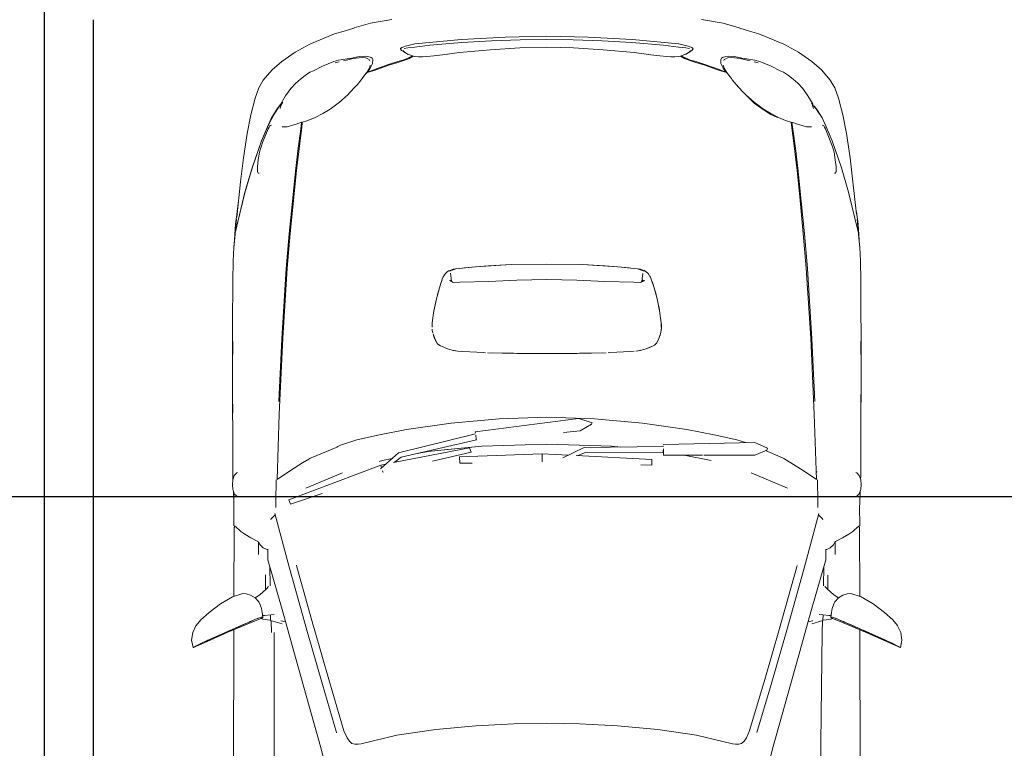
# Model space of a CAD drawing. Units: millimetres. Extents: x 595116 to 630915, y 909473 to 920225.
# Tile 7 of 134: x 629314 to 629404, y 919279 to 919346. Entities that reach past the tile are written whole.
import ezdxf

# ---------------------------------------------------------------- set-up
doc = ezdxf.new("R2010")
doc.units = ezdxf.units.MM
doc.linetypes.add('ACAD_ISO02W100', pattern=[15, 12, -3])
for name, color, linetype, lineweight in [('C-PRKG-VEHI', 8, 'Continuous', 13), ('C-PROP', 7, 'Continuous', 25), ('C-PROP-REF', 240, 'ACAD_ISO02W100', 13), ('Dimension', 3, 'Continuous', 18)]:
    doc.layers.add(name, color=color, linetype=linetype, lineweight=lineweight)
doc.styles.get("Standard").update_dxf_attribs({"font": 'arial.ttf'})
doc.dimstyles.new('ISO-25', dxfattribs={"dimtxt": 9, "dimasz": 6, "dimexe": 1.25, "dimexo": 0.625, "dimtad": 1, "dimlunit": 4, "dimtxsty": 'Standard', "dimcen": 2.5, "dimadec": 0, "dimazin": 0, "dimtfac": 1, "dimtmove": 0, "dimatfit": 3, "dimfxl": 1, "dimarcsym": 0})

# ---------------------------------------------------------------- blocks, each defined once
blk = doc.blocks.new('A$C7ADB3080')
for p, q in [((1725, 1949.3), (1706, 1940.5)), ((1745.5, 1952.4), (1725, 1949.3)), ((1765.9, 1948), (1745.5, 1952.4)), ((1765.8, 1948.2), (1752, 1951)), ((1689.8, 1927.3), (1669.6, 1903.9)), ((1705.6, 1940.3), (1689.8, 1927.3)), ((1706, 1940.5), (1705.6, 1940.3)), ((1750.6, 1917.5), (1752.5, 1921.9)), ((1752.5, 1921.9), (1756.2, 1929.1)), ((1752.5, 1921.9), (1752.5, 1921.9)), ((1765.7, 1947.4), (1752.8, 1918.2)), ((1756.2, 1929.1), (1759.4, 1935.8)), ((1763.8, 1944.5), (1759.4, 1935.8)), ((1759.4, 1935.8), (1762, 1941.3)), ((1759.4, 1935.8), (1759.4, 1935.8)), ((1762, 1941.3), (1763.8, 1944.5)), ((1763.8, 1944.5), (1765, 1946.2)), ((1765, 1946.2), (1765.7, 1947.4)), ((1765.7, 1947.4), (1765.9, 1948)), ((1765.9, 1948), (1765.8, 1948.2)), ((1669.6, 1903.9), (1646.3, 1872.8)), ((1742, 1898.2), (1723, 1855.1)), ((1724.2, 1852.4), (1752.8, 1918.2)), ((1734, 1880.4), (1744, 1903.1)), ((1749.1, 1914.3), (1742, 1898.2)), ((1744, 1903.1), (1746, 1907.5)), ((1746, 1907.5), (1748.3, 1912.5)), ((1748.3, 1912.5), (1750.6, 1917.5)), ((1646.3, 1872.8), (1626.7, 1840.1)), ((1721.5, 1852), (1734, 1880.4)), ((947, 1840.2), (900.9, 1840.1)), ((1014.5, 1840), (947, 1840.2)), ((1724.2, 1852.4), (1697.4, 1788.7)), ((1723, 1855.1), (1704.1, 1812.4)), ((1709.1, 1823.9), (1721.5, 1852)), ((485.6, 1817.6), (419.3, 1809.7)), ((574.5, 1827.8), (485.6, 1817.6)), ((514, 1805.8), (622.7, 1832)), ((568.1, 1827.1), (601.7, 1831.6)), ((596.5, 1830), (587.6, 1828.8)), ((596.5, 1830), (598.5, 1830.3)), ((598.5, 1830.3), (629.8, 1833.4)), ((615.8, 1832.9), (601.7, 1831.6)), ((629.8, 1833.4), (615.8, 1832.9)), ((622.7, 1832), (625.4, 1832.6)), ((625.4, 1832.6), (622.7, 1832)), ((625.4, 1832.6), (627.4, 1832.8)), ((627.4, 1832.8), (625.4, 1832.6)), ((627.4, 1832.8), (629.3, 1833)), ((629.3, 1833), (627.4, 1832.8)), ((630.2, 1833.1), (628.2, 1832.8)), ((644.6, 1834.3), (629.8, 1833.4)), ((666, 1836.1), (630.2, 1833.1)), ((702.2, 1838.3), (666, 1836.1)), ((702.2, 1838.3), (704.4, 1838.4)), ((755.9, 1839.2), (704.4, 1838.4)), ((755.9, 1839.2), (789.1, 1839)), ((846.4, 1839.7), (789.1, 1839)), ((900.9, 1840.1), (846.4, 1839.7)), ((998.4, 1839.9), (923, 1839.2)), ((998.4, 1839.9), (1014.5, 1840)), ((1066.5, 1839.8), (1014.5, 1840)), ((1117.5, 1839.5), (1066.5, 1839.8)), ((1120.4, 1839.3), (1070.3, 1839.6)), ((1164.2, 1839.3), (1117.5, 1839.5)), ((1120.4, 1839.3), (1164.2, 1839.1)), ((1164.2, 1839.1), (1164.1, 1839.1)), ((1186, 1839.2), (1164.2, 1839.3)), ((1211.9, 1839.1), (1164.4, 1839.2)), ((1256.2, 1839), (1211.9, 1839.1)), ((1295.5, 1839), (1256.2, 1839)), ((1284.8, 1825.7), (1285.6, 1828.2)), ((1285.6, 1828.2), (1292.6, 1835.1)), ((1292.6, 1835.1), (1302.3, 1838.5)), ((1295.5, 1839), (1302.9, 1838.7)), ((1302.3, 1838.5), (1304.4, 1839)), ((1304.4, 1839), (1317.7, 1840)), ((1331.1, 1839.1), (1317.7, 1840)), ((1331.1, 1839.1), (1333.2, 1838.5)), ((1342.9, 1835.1), (1333.2, 1838.5)), ((1336.7, 1837.3), (1371.1, 1836.1)), ((1349.8, 1828.2), (1342.9, 1835.1)), ((1350.6, 1825.4), (1349.8, 1828.2)), ((1371.1, 1836.1), (1377.3, 1836)), ((1377.3, 1836), (1430.5, 1836.5)), ((1434.1, 1830.8), (1430.5, 1836.5)), ((1433.4, 1831.8), (1433.4, 1833.5)), ((1433.4, 1833.5), (1433.5, 1833.5)), ((1433.5, 1833.5), (1433.6, 1833.6)), ((1435.6, 1835.7), (1433.6, 1833.6)), ((1445.2, 1818.8), (1434.1, 1830.8)), ((1435.6, 1835.7), (1437, 1835.7)), ((1437, 1835.7), (1625.4, 1836.2)), ((1445.7, 1818.2), (1445.2, 1818.8)), ((1446.6, 1816.9), (1445.7, 1818.2)), ((1453.9, 1805.9), (1446.6, 1816.9)), ((1626.7, 1840.1), (1617.6, 1812)), ((1699.6, 1802.3), (1709.1, 1823.9)), ((1717.5, 1836.5), (2187.9, 1837.4)), ((300.5, 1789.8), (255.3, 1777.9)), ((352.3, 1799.8), (300.5, 1789.8)), ((419.3, 1809.7), (352.3, 1799.8)), ((372.4, 1760.5), (446.6, 1786.3)), ((446.6, 1786.3), (372.4, 1760.5)), ((446.6, 1786.3), (514, 1805.8)), ((514, 1805.8), (446.6, 1786.3)), ((1464, 1789.1), (1453.9, 1805.9)), ((1474.9, 1770), (1464, 1789.1)), ((1617.6, 1812), (1618.4, 1802.1)), ((1618.4, 1802.1), (1622.1, 1790.1)), ((1622.1, 1790.1), (1629.3, 1778)), ((1697.4, 1788.7), (1685.2, 1759.7)), ((1694.1, 1789.9), (1688.5, 1776.5)), ((1691.4, 1783.7), (1694.6, 1791)), ((1691.4, 1783.7), (1694.1, 1789.9)), ((1704.1, 1812.4), (1694.1, 1789.9)), ((1694.1, 1789.9), (1694.6, 1791)), ((1694.6, 1791), (1695.1, 1792.1)), ((1695.1, 1792.1), (1695.6, 1793.4)), ((1695.6, 1793.4), (1696.2, 1794.5)), ((1696.2, 1794.5), (1697.1, 1796.7)), ((1697.1, 1796.7), (1698.1, 1798.8)), ((1698.1, 1798.8), (1698.9, 1800.7)), ((1698.9, 1800.7), (1699.6, 1802.3)), ((227, 1767.4), (205.8, 1755.4)), ((255.3, 1777.9), (227, 1767.4)), ((327.4, 1741.3), (372.4, 1760.5)), ((372.4, 1760.5), (327.4, 1741.3)), ((385.9, 1760.4), (377.1, 1757.2)), ((391.9, 1762.5), (385.9, 1760.4)), ((396.8, 1764.1), (391.9, 1762.5)), ((403.1, 1765.7), (396.8, 1764.1)), ((424.7, 1769.2), (403.1, 1765.7)), ((443.9, 1771.4), (424.7, 1769.2)), ((457.6, 1771.3), (443.9, 1771.4)), ((461, 1769.1), (457.6, 1771.3)), ((461.4, 1766.7), (461, 1769.1)), ((1475.5, 1768.9), (1474.9, 1770)), ((1510, 1768.4), (1475.5, 1768.9)), ((1476.3, 1768.3), (1475.5, 1768.9)), ((1483.6, 1764.1), (1476.3, 1768.3)), ((1491.8, 1755.3), (1483.6, 1764.1)), ((1620.9, 1764.8), (1604.9, 1746.4)), ((1629.8, 1777.6), (1620.9, 1764.8)), ((1629.3, 1778), (1640.8, 1767.9)), ((1640.8, 1767.9), (1649.1, 1763.8)), ((1649.1, 1763.8), (1658.9, 1760.6)), ((1658.9, 1760.6), (1670.1, 1758.3)), ((1683.2, 1763.2), (1682.2, 1758.7)), ((1682.2, 1758.7), (1682.5, 1760.9)), ((1682.5, 1760.9), (1683.2, 1763.2)), ((1688.5, 1776.5), (1683.2, 1763.2)), ((1683.2, 1763.2), (1685.6, 1769.3)), ((1684, 1757.5), (1685.2, 1759.7)), ((1685.2, 1759.7), (1684.6, 1758.5)), ((1685.6, 1769.3), (1688.5, 1776.5)), ((1688, 1756.4), (1686.5, 1762.7)), ((1688.5, 1776.5), (1691.4, 1783.7)), ((205.8, 1755.4), (177.4, 1731.2)), ((296.4, 1724.9), (308.8, 1733)), ((308.8, 1733), (296.4, 1724.9)), ((308.8, 1733), (327.4, 1741.3)), ((327.4, 1741.3), (308.8, 1733)), ((329.5, 1733), (330.6, 1736)), ((331.4, 1737.3), (330.6, 1736)), ((334.6, 1739.6), (331.4, 1737.3)), ((339.6, 1742.2), (334.6, 1739.6)), ((377.1, 1757.2), (339.6, 1742.2)), ((1411.9, 1733.6), (1401.3, 1722.8)), ((1414.5, 1734.8), (1411.9, 1733.6)), ((1496.1, 1745.8), (1491.8, 1755.3)), ((1496.8, 1742), (1496.1, 1745.8)), ((1524.8, 1743.1), (1496.6, 1743.1)), ((1661.6, 1703.9), (1524.8, 1743.1)), ((1596, 1736.9), (1543.4, 1737.8)), ((1607.1, 1748.9), (1567, 1748.9)), ((1604.9, 1746.4), (1597.9, 1740.6)), ((1670.1, 1758.3), (1682.7, 1756.6)), ((1675.3, 1725.1), (1675.9, 1734.9)), ((1675.9, 1734.9), (1677.6, 1752)), ((1692, 1735.3), (1676, 1735.6)), ((1677.6, 1752), (1678.3, 1757.2)), ((1682.3, 1757.1), (1682.2, 1758.7)), ((1682.2, 1758.7), (1682.7, 1756.6)), ((1682.7, 1756.6), (1682.3, 1757.1)), ((1682.7, 1756.6), (1684, 1757.5)), ((1683.3, 1756.9), (1682.7, 1756.6)), ((1684, 1757.5), (1683.3, 1756.9)), ((1684.6, 1758.5), (1684, 1757.5)), ((1690, 1743.9), (1688, 1756.4)), ((1690.8, 1736.6), (1690, 1743.9)), ((1690.9, 1735.3), (1690.8, 1736.6)), ((1700.5, 1704.4), (1692, 1735.3)), ((1724.4, 1733.1), (1692.5, 1733.5)), ((2375.6, 1724.9), (1724.4, 1733.1)), ((177.4, 1731.2), (154.5, 1704.8)), ((248.7, 1693.9), (272.8, 1708.2)), ((272.8, 1708.2), (248.7, 1693.9)), ((274.1, 1706.2), (268.7, 1703.4)), ((278, 1711.4), (275.4, 1709.5)), ((275.5, 1706.9), (283.4, 1709.5)), ((276.7, 1711.4), (284.8, 1717.1)), ((287.5, 1718), (278, 1711.4)), ((284.8, 1717.1), (296.4, 1724.9)), ((298.6, 1725.5), (287.5, 1718)), ((1124.1, 1711.4), (915.2, 1701.7)), ((917.2, 1704.7), (1089.1, 1712.9)), ((1303.7, 1717.2), (1124.1, 1711.4)), ((1279.1, 1680.6), (1303.7, 1717.2)), ((1284, 1719.6), (1282.1, 1716.5)), ((1304.9, 1720.3), (1365.2, 1721)), ((1365.2, 1721), (1380.7, 1721.1)), ((1397.7, 1723.7), (1548.1, 1683.7)), ((1692.9, 1707.2), (1693, 1706.9)), ((1693, 1706.9), (1695.6, 1694.4)), ((128.8, 1668.1), (153.9, 1704.5)), ((214.1, 1665.8), (228.3, 1679.7)), ((228.3, 1679.7), (214.1, 1665.8)), ((228.3, 1679.7), (248.7, 1693.9)), ((248.7, 1693.9), (228.3, 1679.7)), ((330.2, 1678.1), (326.2, 1665.2)), ((333.4, 1690.2), (330.2, 1678.1)), ((333.6, 1703.6), (333.4, 1690.2)), ((627.3, 1681.1), (536.8, 1672.6)), ((538.3, 1675.5), (628.6, 1684.1)), ((722.4, 1689.2), (627.3, 1681.1)), ((628.6, 1684.1), (723.6, 1692.3)), ((915.2, 1701.7), (722.4, 1689.2)), ((723.6, 1692.3), (917.2, 1704.7)), ((1257.7, 1647.2), (1279.1, 1680.6)), ((1548.1, 1683.7), (1718.6, 1636)), ((1799.6, 1665.1), (1661.6, 1703.9)), ((106.5, 1627.7), (128.8, 1668.1)), ((192.9, 1640.1), (202.7, 1653)), ((202.7, 1653), (192.9, 1640.1)), ((202.7, 1653), (214.1, 1665.8)), ((214.1, 1665.8), (202.7, 1653)), ((326.2, 1665.2), (320.7, 1650)), ((320.7, 1650), (340.1, 1652.4)), ((343.5, 1650.7), (321.3, 1648)), ((340.1, 1652.4), (392.9, 1659.3)), ((371.1, 1654.1), (343.5, 1650.7)), ((401.8, 1657.9), (371.1, 1654.1)), ((392.9, 1659.3), (455.7, 1666.7)), ((454.1, 1664), (401.8, 1657.9)), ((536.8, 1672.6), (454.1, 1664)), ((455.7, 1666.7), (538.2, 1675.4)), ((538.2, 1675.4), (538.2, 1675.4)), ((538.3, 1675.5), (538.3, 1675.5)), ((1543.7, 1663.2), (1540.2, 1664.1)), ((1714, 1615.6), (1543.7, 1663.2)), ((1927.3, 1629.4), (1799.6, 1665.1)), ((78.4, 1559.2), (106.5, 1627.7)), ((179.4, 1617.7), (183.6, 1626.9)), ((183.6, 1626.9), (179.4, 1617.7)), ((183.6, 1626.9), (192.9, 1640.1)), ((192.9, 1640.1), (183.6, 1626.9)), ((308, 1612.7), (316.4, 1632.4)), ((316.4, 1632.4), (321.9, 1649.9)), ((320.7, 1649.8), (320.7, 1650)), ((320.7, 1650), (321, 1650)), ((321.9, 1649.9), (322, 1650.2)), ((1224.6, 1577), (1244.4, 1624.1)), ((1244.4, 1624.1), (1245.8, 1627.5)), ((1245.8, 1627.5), (1247.6, 1630.5)), ((1247.6, 1630.5), (1257.7, 1647.2)), ((1285.5, 1538), (1327.9, 1638.1)), ((1718.6, 1636), (1868.2, 1592.8)), ((2038.3, 1598.2), (1927.3, 1629.4)), ((166.6, 1592.6), (179.4, 1617.7)), ((179.4, 1617.7), (166.6, 1592.6)), ((297.6, 1592.1), (308, 1612.7)), ((299.6, 1592.1), (308.6, 1609.9)), ((1714, 1615.6), (1708.7, 1617.1)), ((1860.7, 1573.2), (1714, 1615.6)), ((2088.8, 1585.4), (2038.3, 1598.2)), ((154.1, 1561.6), (166.6, 1592.6)), ((166.6, 1592.6), (154.1, 1561.6)), ((265.7, 1546.2), (285.2, 1572)), ((284.8, 1567.7), (299.6, 1592.1)), ((285.2, 1572), (297.6, 1592.1)), ((1201.9, 1547.7), (1217.9, 1583.1)), ((1223, 1580.9), (1217.9, 1583.1)), ((1236.7, 1548.1), (1223, 1580.9)), ((1863.6, 1572.4), (1860.7, 1573.2)), ((1994.6, 1533.7), (1863.6, 1572.4)), ((1868.2, 1592.8), (2000, 1553.9)), ((70.3, 1532.9), (78.4, 1559.2)), ((147.2, 1525.2), (150.6, 1548.3)), ((150.6, 1548.3), (147.2, 1525.2)), ((150.6, 1548.3), (154.1, 1561.6)), ((154.1, 1561.6), (150.6, 1548.3)), ((158.2, 1557.5), (154.9, 1546.4)), ((245.7, 1523), (265.7, 1546.2)), ((268.5, 1546.6), (247.9, 1525.1)), ((284.8, 1567.7), (268.5, 1546.6)), ((284.8, 1567.7), (284.7, 1567.6)), ((1207.6, 1296.6), (1201.9, 1547.7)), ((1236.9, 1407.5), (1236.7, 1548.1)), ((62.1, 1506.7), (66.6, 1521)), ((66.6, 1521), (70.3, 1532.9)), ((144.6, 1512.1), (147.2, 1525.2)), ((147.2, 1525.2), (144.6, 1512.1)), ((150.3, 1526.6), (145.9, 1508)), ((152.2, 1535), (150.3, 1526.6)), ((247.9, 1525.1), (237.6, 1515.3)), ((1195.1, 1498.2), (1202.5, 1522)), ((1285.3, 1537.6), (1285.5, 1538)), ((2014.5, 1525), (1992.9, 1534.5)), ((2023.9, 1518.6), (2014.5, 1525)), ((2029.9, 1511.6), (2023.9, 1518.6)), ((61.6, 1504.8), (48.4, 1460.7)), ((61.6, 1504.8), (62.1, 1506.7)), ((139.4, 1475.5), (140.7, 1492.2)), ((140.7, 1492.2), (139.4, 1475.5)), ((140.7, 1492.2), (144.6, 1512.1)), ((144.6, 1512.1), (140.7, 1492.2)), ((145.9, 1508), (143.4, 1483.5)), ((217.4, 1496.7), (204.5, 1486.1)), ((225.8, 1504.4), (217.4, 1496.7)), ((237.6, 1515.3), (225.8, 1504.4)), ((1180.7, 1436.4), (1195.1, 1498.2)), ((2031.7, 1503.8), (2029.9, 1511.6)), ((2030.9, 1486.7), (2032.1, 1494.6)), ((2032.1, 1494.6), (2031.7, 1503.8)), ((140.1, 1468.1), (139.4, 1475.5)), ((139.4, 1475.5), (140.1, 1468.1)), ((143.2, 1458.9), (140.1, 1468.1)), ((140.1, 1468.1), (143.2, 1458.9)), ((143.4, 1483.5), (144.5, 1474.1)), ((144.5, 1474.1), (146.2, 1469.1)), ((146.5, 1468.2), (149.1, 1464)), ((149.1, 1464), (151.7, 1462.6)), ((164.5, 1461.2), (172.2, 1463.8)), ((172, 1462.5), (184.5, 1470.4)), ((172.2, 1463.8), (181.7, 1469.2)), ((183.7, 1468.4), (172.4, 1461.2)), ((172.4, 1461.2), (183.7, 1468.4)), ((174.2, 1464.8), (173.9, 1464.7)), ((174.8, 1465.1), (174.2, 1464.8)), ((176.1, 1450.1), (183.7, 1468.4)), ((184.7, 1470.2), (178.9, 1450.6)), ((181.7, 1469.2), (186.7, 1472.5)), ((183.5, 1468), (184.1, 1468.1)), ((183.7, 1468.4), (184.5, 1470.4)), ((184, 1469.2), (184.5, 1469.5)), ((184.1, 1469.5), (184.6, 1469.7)), ((184.5, 1470.4), (185.1, 1470.6)), ((187.2, 1473), (184.7, 1470.2)), ((201, 1483.7), (187.2, 1473)), ((204.5, 1486.1), (201, 1483.7)), ((2007.4, 1388.1), (2030.9, 1486.7)), ((48.4, 1460.7), (38.4, 1401.7)), ((145, 1456.1), (143.2, 1458.9)), ((143.2, 1458.9), (145, 1456.1)), ((148.9, 1454.2), (145, 1456.1)), ((145, 1456.1), (148.9, 1454.2)), ((160, 1454.9), (148.9, 1454.2)), ((148.9, 1454.2), (160, 1454.9)), ((172.4, 1461.2), (160, 1454.9)), ((160, 1454.9), (172.4, 1461.2)), ((162.7, 1410.7), (176.1, 1450.1)), ((178.9, 1450.6), (164.5, 1410.7)), ((1166.8, 1361.5), (1180.7, 1436.4)), ((154.5, 1385.6), (162.7, 1410.7)), ((164.5, 1410.7), (156.5, 1386)), ((1237, 1353.9), (1251.4, 1427.7)), ((150.2, 1371.5), (154.5, 1385.6)), ((156.5, 1386), (151.3, 1369.4)), ((1237.1, 1297.2), (1236.9, 1403.7)), ((1991.5, 1281.2), (2007.4, 1388.1)), ((105.3, 1338.7), (112.3, 1364.4)), ((112.3, 1364.4), (105.3, 1338.7)), ((112.3, 1364.4), (113.8, 1369.4)), ((113.8, 1369.4), (112.3, 1364.4)), ((113.8, 1369.4), (115.5, 1374.4)), ((115.5, 1374.4), (113.8, 1369.4)), ((117, 1357.9), (114.6, 1338.6)), ((115.5, 1374.4), (118, 1378)), ((118, 1378), (115.5, 1374.4)), ((118.7, 1368.1), (117, 1357.9)), ((118, 1378), (119.5, 1378.4)), ((119.5, 1378.4), (118, 1378)), ((119.5, 1378.4), (123.8, 1375.2)), ((123.8, 1375.2), (119.5, 1378.4)), ((123.7, 1371.6), (127.9, 1368.1)), ((123.8, 1375.2), (127.7, 1369.2)), ((127.7, 1369.2), (123.8, 1375.2)), ((127.7, 1369.2), (133.5, 1360.1)), ((133.5, 1360.1), (127.7, 1369.2)), ((127.9, 1368.1), (131.7, 1361.7)), ((131.7, 1361.7), (134.5, 1357.5)), ((133.5, 1360.1), (137.9, 1348.2)), ((137.9, 1348.2), (133.5, 1360.1)), ((138.7, 1345.5), (145.3, 1358.5)), ((145.6, 1354.8), (139.2, 1343.6)), ((145.3, 1358.5), (150.2, 1371.5)), ((151.3, 1369.4), (145.6, 1354.8)), ((1149.4, 1239.2), (1166.8, 1361.5)), ((93.5, 1210.7), (105.3, 1338.7)), ((105.3, 1338.7), (93.5, 1210.7)), ((114.6, 1338.6), (109.6, 1297.4)), ((137.9, 1348.2), (138.7, 1345.5)), ((138.7, 1345.5), (137.9, 1348.2)), ((140.3, 1345.5), (138.7, 1345.5)), ((139.2, 1343.6), (140.6, 1338.5)), ((140.1, 1345.5), (140.2, 1345.3)), ((140.6, 1338.5), (141.3, 1328.4)), ((141.3, 1328.4), (141, 1317.4)), ((140.1, 1305.8), (138.4, 1286.6)), ((141, 1317.4), (140.1, 1305.8)), ((109.6, 1297.4), (102.1, 1210)), ((138.4, 1286.6), (135.7, 1262.5)), ((807.2, 1279.5), (776.6, 1271.5)), ((783.2, 1273.2), (791.1, 1275.6)), ((791.1, 1275.6), (800.2, 1277.7)), ((840.1, 1286.2), (807.2, 1279.5)), ((816.8, 1281.5), (831.5, 1284.8)), ((831.5, 1284.8), (838.3, 1285.8)), ((873.1, 1290.9), (840.1, 1286.2)), ((888.8, 1291.1), (873.1, 1290.9)), ((873.2, 1290.9), (876.6, 1291.3)), ((876.6, 1291.3), (884.9, 1291)), ((903.4, 1288.7), (888.8, 1291.1)), ((890.4, 1290.8), (894.1, 1290.7)), ((894.1, 1290.7), (899.9, 1289.3)), ((916.5, 1284.3), (903.4, 1288.7)), ((906.8, 1287.6), (908, 1287.3)), ((908, 1287.3), (916.4, 1284.4)), ((916.4, 1284.4), (923.9, 1280.5)), ((927.7, 1278.5), (916.5, 1284.3)), ((923.9, 1280.5), (924.7, 1280.1)), ((931.6, 1275.4), (927.7, 1278.5)), ((928.5, 1277.9), (929.6, 1277.2)), ((929.6, 1277.2), (930.1, 1276.6)), ((934.3, 1272), (931.6, 1275.4)), ((936.3, 1268.2), (934.3, 1272)), ((1207.6, 1296.6), (1209.6, 1296.4)), ((1215.8, 1078.8), (1213.2, 1296.7)), ((1227.6, 1296), (1219.5, 1296.9)), ((1222.6, 1296.6), (1237.1, 1297.2)), ((1226.3, 1296.1), (1226.4, 1296.8)), ((1230.4, 1295.7), (1227.6, 1296)), ((1229.7, 1083), (1230.4, 1295.7)), ((1981.3, 1170.9), (1991.5, 1281.2)), ((135.7, 1262.5), (129.8, 1216.2)), ((732.6, 1249.6), (728.6, 1244.4)), ((737.5, 1254.5), (732.6, 1249.6)), ((733.1, 1250.3), (733, 1250.1)), ((733.3, 1250.3), (733.1, 1250.3)), ((743.3, 1258.9), (737.5, 1254.5)), ((750.3, 1262.4), (743.3, 1258.9)), ((744.9, 1259.7), (745.5, 1260.1)), ((745.5, 1260.1), (746.8, 1260.6)), ((776.6, 1271.5), (750.3, 1262.4)), ((755.5, 1264.2), (760.9, 1266.4)), ((756.6, 1246), (761.8, 1233.7)), ((760.9, 1266.4), (769.9, 1269.2)), ((935.3, 1270), (936.3, 1268.7)), ((936.3, 1268.7), (941.9, 1256.9)), ((938.5, 1264), (936.3, 1268.2)), ((944.5, 1249.5), (938.5, 1264)), ((941.9, 1256.9), (943, 1253.2)), ((948.4, 1236.1), (944.5, 1249.5)), ((1248.6, 1264.5), (1238.1, 1056.7)), ((1264.7, 1265), (1248.6, 1264.5)), ((1263.8, 1234.3), (1264.7, 1265)), ((724, 1225.9), (718.5, 1171.5)), ((730.7, 1243.7), (724, 1225.9)), ((724.5, 1227.4), (725.2, 1233.3)), ((725.2, 1233.3), (729.7, 1243.8)), ((728.6, 1244.4), (730.5, 1243.3)), ((758.8, 1237.8), (737.6, 1240.5)), ((755.9, 1240.9), (761.1, 1235.4)), ((755.9, 1240.9), (755.9, 1240.9)), ((756.8, 1244), (759.3, 1239.6)), ((756.8, 1244), (756.8, 1244)), ((761.5, 1215.3), (761.8, 1234)), ((950.5, 1221.1), (948.4, 1236.1)), ((948.6, 1234.4), (949, 1233.2)), ((949, 1233.2), (949.6, 1227.7)), ((1137.2, 1107.4), (1149.4, 1239.2)), ((86.9, 1090.2), (93.5, 1210.7)), ((93.5, 1210.7), (86.9, 1090.2)), ((102.1, 1210), (97.3, 1128.3)), ((129.8, 1216.2), (121.7, 1131.5)), ((718.5, 1171.7), (721.7, 1202.7)), ((721.7, 1202.7), (721.7, 1203)), ((761.5, 1215.3), (759.2, 1135.8)), ((950.8, 1216.3), (951.9, 1206.7)), ((951.9, 1206.7), (954.9, 1149.6)), ((718.5, 1171.5), (712.9, 1074.6)), ((716.1, 1136.1), (718.5, 1171.7)), ((1212, 1154.3), (1214.6, 1179.7)), ((1214.6, 1179.7), (1212.1, 1154.5)), ((1976, 1066.4), (1981.3, 1170.9)), ((954.9, 1149.6), (955.1, 1144.6)), ((956.9, 1058.9), (955.4, 1139.5)), ((1212.1, 1154.5), (1207, 976.2)), ((1207, 976.2), (1212, 1154.3)), ((97.3, 1128.3), (94.3, 1048.9)), ((121.7, 1131.5), (116.6, 1049.9)), ((712.8, 1074.5), (716.1, 1136.1)), ((759.2, 1135.8), (755.9, 1058.6)), ((955.6, 1128.3), (956.8, 1091.9)), ((84.7, 976.2), (86.9, 1090.2)), ((86.9, 1090.2), (84.7, 976.2)), ((956.8, 1091.9), (956.8, 1066.5)), ((1132.6, 976.2), (1137.2, 1107.4)), ((1135.7, 1064.3), (1148.4, 1101)), ((1152, 1099.3), (1148.4, 1101)), ((1169.8, 1068.2), (1152, 1099.3)), ((1238.3, 1061.1), (1229.7, 1083)), ((712.9, 1074.6), (711.4, 976.2)), ((711.4, 976.2), (712.8, 1074.5)), ((755.9, 1058.6), (754.2, 976.2)), ((957.1, 976.2), (956.9, 1058.9)), ((1172.6, 779.7), (1135.7, 1063.8)), ((1174.9, 1022.3), (1169.8, 1068.2)), ((1243.9, 1020.7), (1215.8, 1078.8)), ((1974.1, 976.2), (1976, 1066.4)), ((94.3, 1048.9), (93.3, 976.2)), ((116.6, 1049.9), (114.8, 976.2)), ((1237, 1034.9), (1233.4, 963.6)), ((1243.9, 1020.7), (1244.3, 1020.7)), ((86.9, 862.1), (84.7, 976.2)), ((84.7, 976.2), (86.9, 862.1)), ((93.3, 976.2), (94.3, 903.4)), ((114.8, 976.2), (116.6, 902.5)), ((711.4, 976.2), (712.9, 877.9)), ((712.8, 877.9), (711.4, 976.2)), ((754.2, 976.2), (755.9, 893.8)), ((956.9, 893.5), (957.1, 976.2)), ((1137.2, 845), (1132.6, 976.2)), ((1212, 798.1), (1207, 976.2)), ((1207, 976.2), (1212.1, 797.9)), ((1976, 886), (1974.1, 976.2)), ((1233.4, 963.6), (1242, 736.5)), ((1251.9, 963.2), (1233.4, 963.6)), ((1254.9, 963.3), (1251.9, 963.2)), ((94.3, 903.4), (97.3, 824.1)), ((116.6, 902.5), (121.7, 820.9)), ((755.9, 893.8), (759.2, 816.6)), ((955.4, 812.9), (956.9, 893.5)), ((716.1, 816.3), (712.8, 877.9)), ((712.9, 877.9), (718.6, 779.9)), ((956.8, 885.8), (956.8, 860.5)), ((1981.3, 781.5), (1976, 886)), ((93.5, 741.7), (86.9, 862.1)), ((86.9, 862.1), (93.5, 741.7)), ((956.8, 860.5), (955.6, 824.1)), ((1149.4, 713.2), (1137.2, 845)), ((97.3, 824.1), (102.1, 742.4)), ((121.7, 820.9), (129.8, 736.1)), ((718.5, 780.7), (716.1, 816.3)), ((759.2, 816.6), (761.5, 737.1)), ((954.9, 802.8), (951.9, 745.7)), ((955.1, 807.8), (954.9, 802.8)), ((1227, 649.4), (1212, 798.1)), ((1212.1, 797.9), (1222.5, 694.4)), ((721.6, 749.8), (718.5, 780.7)), ((718.6, 779.9), (724, 726.5)), ((1172.6, 779.7), (1175.9, 779.9)), ((1230.5, 568.5), (1178, 780.4)), ((1193.1, 782.3), (1182.2, 781)), ((1193.9, 782.6), (1193.1, 782.3)), ((1242.6, 576.1), (1194.9, 782.6)), ((1228.9, 768.7), (1217.2, 764.2)), ((1217.2, 764.2), (1257.5, 555)), ((1253.7, 662.2), (1228.9, 768.7)), ((1259.1, 737.2), (1258.7, 771.2)), ((1991.5, 671.2), (1981.3, 781.5)), ((105.3, 613.6), (93.5, 741.7)), ((93.5, 741.7), (105.3, 613.6)), ((102.1, 742.4), (109.6, 654.9)), ((129.8, 736.1), (135.7, 689.9)), ((761.5, 737.1), (761.8, 718.7)), ((948.4, 716.3), (950.5, 731.3)), ((951.9, 745.7), (950.5, 731.3)), ((1242, 736.5), (1258.1, 737)), ((1259.1, 737.2), (1258.1, 737)), ((724, 726.5), (730.7, 708.6)), ((725.2, 719.1), (724.5, 725)), ((729.7, 708.6), (725.2, 719.1)), ((730.5, 709), (728.6, 708)), ((728.6, 708), (732.6, 702.8)), ((758.4, 714.2), (736.5, 711.7)), ((755.9, 711.5), (761, 717)), ((756.8, 708.4), (761.8, 718.7)), ((944.5, 702.9), (948.4, 716.3)), ((949.6, 724.7), (949, 719.2)), ((1166.8, 590.9), (1149.4, 713.2)), ((135.7, 689.9), (138.4, 665.8)), ((732.6, 702.8), (737.5, 697.9)), ((733, 702.3), (733.1, 702.1)), ((733.1, 702.1), (733.3, 702.1)), ((737.5, 697.9), (743.3, 693.5)), ((743.3, 693.5), (750.3, 690)), ((745.5, 692.3), (744.9, 692.7)), ((746.8, 691.7), (745.5, 692.3)), ((750.3, 690), (776.6, 680.9)), ((760.9, 685.9), (755.5, 688.2)), ((769.9, 683.2), (760.9, 685.9)), ((776.6, 680.9), (807.2, 672.8)), ((791.1, 676.8), (783.2, 679.2)), ((800.2, 674.7), (791.1, 676.8)), ((927.7, 673.9), (931.6, 677)), ((931.6, 677), (936.3, 684.2)), ((936.3, 684.2), (938.5, 688.3)), ((938.5, 688.3), (944.5, 702.9)), ((109.6, 654.9), (114.6, 613.7)), ((138.4, 665.8), (140.1, 646.5)), ((807.2, 672.8), (840.1, 666.2)), ((831.5, 667.6), (816.8, 670.9)), ((838.3, 666.6), (831.5, 667.6)), ((840.1, 666.2), (873.1, 661.5)), ((876.6, 661), (873.2, 661.5)), ((885.2, 661.3), (876.6, 661)), ((894.1, 661.6), (890.2, 661.5)), ((900.1, 663.2), (894.1, 661.6)), ((903.4, 663.7), (916.5, 668.1)), ((908, 665.1), (906.7, 664.8)), ((916.4, 668), (908, 665.1)), ((923.9, 671.8), (916.4, 668)), ((916.5, 668.1), (927.7, 673.9)), ((925.2, 672.6), (923.9, 671.8)), ((1227, 649.8), (1234.6, 610.6)), ((2007.4, 564.3), (1991.5, 671.2)), ((140.1, 646.5), (141, 635)), ((141.3, 624), (140.6, 613.9)), ((141, 635), (141.3, 624)), ((1234.5, 611.2), (1227, 649.4)), ((112.3, 588), (105.3, 613.6)), ((105.3, 613.6), (112.3, 588)), ((114.6, 613.7), (117, 594.4)), ((137.9, 604.2), (133.5, 592.2)), ((133.5, 592.2), (137.9, 604.2)), ((138.7, 606.9), (137.9, 604.2)), ((137.9, 604.2), (138.7, 606.9)), ((145.3, 593.9), (138.7, 606.9)), ((138.7, 606.9), (140.3, 606.9)), ((140.6, 613.9), (139.2, 608.8)), ((139.2, 608.8), (145.6, 597.6)), ((140.2, 607), (140.2, 606.9)), ((145.6, 597.6), (151.3, 583)), ((113.8, 583), (112.3, 588)), ((112.3, 588), (113.8, 583)), ((115.5, 577.9), (113.8, 583)), ((113.8, 583), (115.5, 577.9)), ((118, 574.3), (115.5, 577.9)), ((115.5, 577.9), (118, 574.3)), ((117, 594.4), (118.7, 584.2)), ((119.5, 573.9), (118, 574.3)), ((118, 574.3), (119.5, 573.9)), ((123.8, 577.2), (119.5, 573.9)), ((119.5, 573.9), (123.8, 577.2)), ((127.9, 584.3), (123.7, 580.8)), ((127.7, 583.2), (123.8, 577.2)), ((123.8, 577.2), (127.7, 583.2)), ((133.5, 592.2), (127.7, 583.2)), ((127.7, 583.2), (133.5, 592.2)), ((131.7, 590.6), (127.9, 584.3)), ((134.5, 594.9), (131.7, 590.6)), ((150.2, 580.9), (145.3, 593.9)), ((154.5, 566.8), (150.2, 580.9)), ((151.3, 583), (156.5, 566.4)), ((1180.7, 516), (1166.8, 590.9)), ((1274.5, 519), (1230.5, 568.5)), ((1257.1, 557), (1242.6, 576.1)), ((38.4, 550.7), (48.4, 491.6)), ((162.7, 541.6), (154.5, 566.8)), ((156.5, 566.4), (164.5, 541.7)), ((176.1, 502.3), (162.7, 541.6)), ((164.5, 541.7), (178.9, 501.8)), ((1251.4, 524.6), (1246.3, 550.8)), ((1246.3, 550.8), (1251.4, 524.7)), ((2030.9, 465.7), (2007.4, 564.3)), ((1195.1, 454.2), (1180.7, 516)), ((1251.4, 524.7), (1251.4, 524.6)), ((1254.1, 515.9), (1251.4, 524.6)), ((1261.6, 533.5), (1264.2, 519.8)), ((1271.7, 522.2), (1264.2, 519.8)), ((1264.2, 519.8), (1359.7, 267.1)), ((1274.5, 519), (1275, 519.1)), ((1282.4, 525.7), (1279.7, 524.8)), ((1284.5, 526.7), (1282.4, 525.7)), ((1284.5, 526.7), (1282.4, 525.7)), ((61.8, 446.6), (48.4, 491.6)), ((143.2, 493.4), (140.1, 484.3)), ((140.1, 484.3), (143.2, 493.4)), ((145, 496.2), (143.2, 493.4)), ((143.2, 493.4), (145, 496.2)), ((148.9, 498.2), (145, 496.2)), ((145, 496.2), (148.9, 498.2)), ((149.1, 488.4), (146.5, 484.2)), ((160, 497.5), (148.9, 498.2)), ((148.9, 498.2), (160, 497.5)), ((151.9, 489.8), (149.1, 488.4)), ((172.4, 491.2), (160, 497.5)), ((160, 497.5), (172.4, 491.2)), ((172.2, 488.6), (164.5, 491.2)), ((181.7, 483.1), (172.2, 488.6)), ((183.7, 484), (172.4, 491.2)), ((172.4, 491.2), (183.7, 484)), ((183.7, 484), (176.1, 502.3)), ((178.9, 501.8), (184.7, 482.1)), ((140.1, 484.3), (139.4, 476.9)), ((139.4, 476.9), (140.1, 484.3)), ((139.4, 476.9), (140.7, 460.2)), ((140.7, 460.2), (139.4, 476.9)), ((140.7, 460.2), (144.6, 440.3)), ((144.6, 440.3), (140.7, 460.2)), ((144.5, 478.2), (143.4, 468.8)), ((143.4, 468.8), (145.9, 444.4)), ((146.2, 483.2), (144.5, 478.2)), ((186.8, 479.9), (181.7, 483.1)), ((184.5, 482), (183.7, 484)), ((185.1, 481.8), (184.5, 482)), ((184.7, 482.1), (187.2, 479.3)), ((187.2, 479.3), (201, 468.7)), ((201, 468.7), (204.5, 466.3)), ((204.5, 466.3), (217.4, 455.7)), ((2032.1, 457.8), (2030.9, 465.7)), ((62.1, 445.7), (61.6, 447.5)), ((66.6, 431.3), (62.1, 445.7)), ((144.6, 440.3), (147.2, 427.2)), ((147.2, 427.2), (144.6, 440.3)), ((145.9, 444.4), (150.3, 425.8)), ((217.4, 455.7), (225.8, 447.9)), ((225.8, 447.9), (237.6, 437)), ((237.6, 437), (247.9, 427.3)), ((1209.1, 409.1), (1195.1, 454.2)), ((2014.5, 427.4), (2023.9, 433.8)), ((2023.9, 433.8), (2029.9, 440.8)), ((2029.9, 440.8), (2031.7, 448.5)), ((2031.7, 448.5), (2032.1, 457.8)), ((70.3, 419.5), (66.6, 431.3)), ((78.4, 393.2), (70.3, 419.5)), ((147.2, 427.2), (150.6, 404)), ((150.6, 404), (147.2, 427.2)), ((150.3, 425.8), (152.2, 417.4)), ((154.9, 405.9), (158.1, 394.9)), ((265.7, 406.2), (245.5, 429.5)), ((285.2, 380.4), (265.7, 406.2)), ((1211.1, 405.7), (1209.1, 409.1)), ((1285.5, 414.4), (1285.3, 414.8)), ((1327.9, 314.3), (1285.5, 414.4)), ((1863.6, 380), (1994.8, 418.7)), ((1994.8, 418.7), (2014.5, 427.4)), ((106.5, 324.6), (78.4, 393.2)), ((150.6, 404), (154.1, 390.7)), ((154.1, 390.7), (150.6, 404)), ((154.1, 390.7), (166.6, 359.8)), ((166.6, 359.8), (154.1, 390.7)), ((297.6, 360.3), (285.2, 380.4)), ((1213.2, 402.1), (1211.1, 405.7)), ((1214.7, 399.2), (1213.2, 402.1)), ((1215.6, 397), (1214.7, 399.2)), ((1244.4, 328.3), (1215.6, 397)), ((1714, 336.8), (1860.7, 379.1)), ((1860.7, 379.1), (1863.6, 380)), ((2000, 398.5), (1868.2, 359.6)), ((2000, 398.5), (2000.4, 398.7)), ((166.6, 359.8), (179.4, 334.6)), ((179.4, 334.6), (166.6, 359.8)), ((308, 339.7), (297.6, 360.3)), ((1372.2, 272.1), (1342.5, 359.1)), ((1868.2, 359.6), (1718.6, 316.3)), ((1927.3, 323), (2038.3, 354.2)), ((2038.3, 354.2), (2088.8, 367)), ((179.4, 334.6), (183.6, 325.4)), ((183.6, 325.4), (179.4, 334.6)), ((183.6, 325.4), (192.9, 312.3)), ((192.9, 312.3), (183.6, 325.4)), ((316.4, 319.9), (308, 339.7)), ((1245.8, 324.9), (1244.4, 328.3)), ((1247.6, 321.8), (1245.8, 324.9)), ((1543.7, 289.1), (1708.7, 335.3)), ((1708.7, 335.3), (1714, 336.8)), ((128.8, 284.3), (106.5, 324.6)), ((192.9, 312.3), (202.7, 299.4)), ((202.7, 299.4), (192.9, 312.3)), ((202.7, 299.4), (214.1, 286.6)), ((214.1, 286.6), (202.7, 299.4)), ((321.9, 302.5), (316.4, 319.9)), ((320.7, 302.4), (320.7, 302.6)), ((340.1, 300), (320.7, 302.4)), ((320.7, 302.4), (326.2, 287.1)), ((321, 302.4), (320.7, 302.4)), ((322, 302.2), (321.9, 302.5)), ((323.2, 304.2), (323.4, 304.1)), ((323.9, 302.5), (323.4, 304.1)), ((323.4, 304.1), (343.5, 301.6)), ((324.1, 301.9), (323.9, 302.5)), ((324.8, 302.3), (324, 302.3)), ((326.6, 303.7), (326.9, 302)), ((328.2, 302.2), (326.9, 302.3)), ((328.2, 303.5), (328.2, 302.2)), ((392.9, 293.1), (340.1, 300)), ((343.5, 301.6), (371.1, 298.2)), ((371.1, 298.2), (401.8, 294.5)), ((1257.7, 305.2), (1247.6, 321.8)), ((1279.1, 271.8), (1257.7, 305.2)), ((1328, 314.1), (1327.9, 314.3)), ((1718.6, 316.3), (1548.1, 268.7)), ((1799.6, 287.3), (1927.3, 323)), ((153.9, 247.9), (128.8, 284.3)), ((214.1, 286.6), (228.3, 272.7)), ((228.3, 272.7), (214.1, 286.6)), ((228.3, 272.7), (248.7, 258.4)), ((248.7, 258.4), (228.3, 272.7)), ((326.2, 287.1), (330.2, 274.3)), ((330.2, 274.3), (333.4, 262.2)), ((455.7, 285.7), (392.9, 293.1)), ((401.8, 294.5), (454.1, 288.4)), ((454.1, 288.4), (536.8, 279.7)), ((538.2, 276.9), (455.7, 285.7)), ((536.8, 279.7), (627.3, 271.2)), ((538.2, 276.9), (538.2, 276.9)), ((628.6, 268.2), (538.3, 276.9)), ((538.3, 276.9), (538.3, 276.9)), ((627.3, 271.2), (722.4, 263.1)), ((1303.7, 235.1), (1279.1, 271.8)), ((1359.7, 267.1), (1371.5, 271.7)), ((1372.2, 272.1), (1371.5, 271.7)), ((1539.5, 288), (1543.7, 289.1)), ((1661.6, 248.5), (1799.6, 287.3)), ((156.5, 245), (153.9, 247.9)), ((154, 247.9), (177.4, 221.2)), ((248.7, 258.4), (272.8, 244.2)), ((272.8, 244.2), (248.7, 258.4)), ((273.8, 245.9), (266.3, 250.4)), ((268.3, 249.3), (274.1, 246.2)), ((272.8, 244.2), (273.8, 245.9)), ((274.3, 244.9), (272.8, 244.2)), ((272.8, 244.2), (276.7, 241)), ((276.7, 241), (272.8, 244.2)), ((274.1, 246.2), (277, 244.9)), ((275.5, 245.4), (274.2, 244.9)), ((275.4, 242.9), (274.2, 244.9)), ((283, 243), (275.5, 245.4)), ((333.4, 262.2), (333.6, 248.8)), ((723.6, 260.1), (628.6, 268.2)), ((722.4, 263.1), (915.2, 250.7)), ((917.2, 247.7), (723.6, 260.1)), ((915.2, 250.7), (1124.1, 241)), ((1089.1, 239.4), (917.2, 247.7)), ((1548.1, 268.7), (1397.7, 228.7)), ((1524.8, 209.3), (1661.6, 248.5)), ((1692, 217.1), (1700.7, 248.5)), ((1693, 245.5), (1692.9, 245.3)), ((1695.6, 258), (1693, 245.5)), ((177.4, 221.2), (205.8, 197)), ((275.4, 242.9), (278, 241)), ((276.7, 241), (284.8, 235.3)), ((284.8, 235.3), (276.7, 241)), ((298.6, 226.9), (278, 241)), ((278, 241), (287.5, 234.4)), ((284.8, 235.3), (296.4, 227.4)), ((296.4, 227.4), (284.8, 235.3)), ((287.5, 234.4), (298.6, 226.9)), ((296.4, 227.4), (308.8, 219.4)), ((308.8, 219.4), (296.4, 227.4)), ((327.9, 211.4), (298.6, 226.9)), ((298.6, 226.9), (310.9, 219)), ((308.8, 219.4), (327.4, 211.1)), ((327.4, 211.1), (308.8, 219.4)), ((310.9, 219), (327.9, 211.4)), ((330.6, 216.3), (329.5, 219.4)), ((1089.1, 239.4), (1089.1, 239.4)), ((1124.1, 241), (1303.7, 235.1)), ((1365.2, 231.3), (1304.9, 232.1)), ((1380.7, 231.3), (1365.2, 231.3)), ((1401.3, 229.6), (1411.9, 218.7)), ((1411.9, 218.7), (1414.5, 217.6)), ((1675.9, 217.5), (1675.3, 227.3)), ((1677.6, 200.4), (1675.9, 217.5)), ((1676, 216.8), (1692, 217.1)), ((1690.8, 215.8), (1690.9, 217.1)), ((1692.5, 218.9), (1724.4, 219.2)), ((1724.4, 226.9), (2375.6, 227.4)), ((205.8, 197), (227, 185)), ((327.4, 211.1), (372.4, 191.8)), ((372.4, 191.8), (327.4, 211.1)), ((327.9, 211.4), (374.7, 191.5)), ((330.6, 216.3), (331.4, 215.1)), ((331.4, 215.1), (334.6, 212.8)), ((334.6, 212.8), (339.6, 210.2)), ((339.6, 210.2), (377.1, 195.2)), ((372.4, 191.8), (446.6, 166.1)), ((446.6, 166.1), (372.4, 191.8)), ((374.7, 191.5), (447.7, 166.2)), ((377.1, 195.2), (385.9, 191.9)), ((385.9, 191.9), (391.9, 189.9)), ((391.9, 189.9), (396.8, 188.3)), ((1483.6, 188.2), (1491.8, 197.1)), ((1491.8, 197.1), (1496.1, 206.6)), ((1496.1, 206.6), (1496.8, 210.3)), ((1496.6, 209.3), (1524.8, 209.3)), ((1543.4, 214.6), (1596, 215.5)), ((1566.6, 203.4), (1607.1, 203.4)), ((1598, 211.8), (1604.9, 206)), ((1604.9, 206), (1620.9, 187.6)), ((1658.9, 191.7), (1649.1, 188.6)), ((1670.1, 194.1), (1658.9, 191.7)), ((1682.7, 195.8), (1670.1, 194.1)), ((1678.3, 195.2), (1677.6, 200.4)), ((1682.7, 195.8), (1682.2, 193.7)), ((1682.2, 193.7), (1682.3, 195.3)), ((1682.5, 191.5), (1682.2, 193.7)), ((1682.2, 193.7), (1683.2, 189.1)), ((1682.3, 195.3), (1682.7, 195.8)), ((1683.2, 189.1), (1682.5, 191.5)), ((1682.7, 195.8), (1683.3, 195.5)), ((1684, 194.8), (1682.7, 195.8)), ((1683.3, 195.5), (1684, 194.8)), ((1684, 194.8), (1684.6, 193.9)), ((1685.2, 192.7), (1684, 194.8)), ((1684.6, 193.9), (1685.2, 192.7)), ((1685.2, 192.7), (1697.4, 163.7)), ((1686.5, 189.6), (1688, 196)), ((1688, 196), (1690, 208.5)), ((1690, 208.5), (1690.8, 215.8)), ((227, 185), (255.3, 174.5)), ((255.3, 174.5), (300.5, 162.6)), ((300.5, 162.6), (352.3, 152.6)), ((396.8, 188.3), (403.1, 186.6)), ((403.1, 186.6), (424.7, 183.2)), ((424.7, 183.2), (443.9, 181)), ((443.9, 181), (457.6, 181.1)), ((446.6, 166.1), (514, 146.6)), ((514, 146.6), (446.6, 166.1)), ((447.7, 166.2), (515, 146.7)), ((457.6, 181.1), (461, 183.3)), ((461, 183.3), (461.4, 185.7)), ((1453.9, 146.5), (1464, 163.2)), ((1464, 163.2), (1474.9, 182.4)), ((1474.9, 182.4), (1475.5, 183.5)), ((1475.5, 183.5), (1476.3, 184.1)), ((1475.5, 183.5), (1510, 183.9)), ((1476.3, 184.1), (1483.6, 188.2)), ((1620.9, 187.6), (1629.8, 174.8)), ((1629.3, 174.4), (1622.1, 162.3)), ((1640.8, 184.4), (1629.3, 174.4)), ((1649.1, 188.6), (1640.8, 184.4)), ((1685.6, 183), (1683.2, 189.1)), ((1683.2, 189.1), (1688.5, 175.8)), ((1688.5, 175.8), (1685.6, 183)), ((1691.4, 168.6), (1688.5, 175.8)), ((1688.5, 175.8), (1694.1, 162.5)), ((1694.6, 161.4), (1691.4, 168.6)), ((1694.1, 162.5), (1691.4, 168.6)), ((1694.6, 161.4), (1694.1, 162.5)), ((1694.1, 162.5), (1704.1, 140)), ((1697.4, 163.7), (1724.2, 100)), ((352.3, 152.6), (419.3, 142.7)), ((419.3, 142.7), (485.6, 134.8)), ((514, 146.6), (622.7, 120.4)), ((622.7, 120.4), (514, 146.6)), ((515, 146.7), (625.4, 120.1)), ((515, 146.7), (515, 146.7)), ((1445.7, 134.2), (1446.6, 135.5)), ((1446.6, 135.5), (1453.9, 146.5)), ((1618.4, 150.3), (1617.6, 140.4)), ((1617.6, 140.4), (1626.7, 112.3)), ((1622.1, 162.3), (1618.4, 150.3)), ((1695.1, 160.2), (1694.6, 161.4)), ((1695.6, 159), (1695.1, 160.2)), ((1696.2, 157.8), (1695.6, 159)), ((1697.1, 155.6), (1696.2, 157.8)), ((1698.1, 153.6), (1697.1, 155.6)), ((1698.9, 151.7), (1698.1, 153.6)), ((1699.6, 150.1), (1698.9, 151.7)), ((1709.1, 128.5), (1699.6, 150.1)), ((1704.1, 140), (1723, 97.3)), ((485.6, 134.8), (582.2, 123.9)), ((529.7, 129.8), (574.5, 124.6)), ((568.1, 125.2), (562.5, 126)), ((601.7, 120.8), (568.1, 125.2)), ((587.6, 123.6), (596.5, 122.4)), ((598.5, 122.1), (596.5, 122.4)), ((598.5, 122.1), (627.4, 119.5)), ((601.7, 120.8), (615.8, 119.5)), ((615.8, 119.5), (629.8, 119)), ((622.7, 120.4), (625.4, 119.8)), ((625.4, 119.8), (622.7, 120.4)), ((625.4, 120.2), (625.4, 120.1)), ((625.4, 120.1), (628.2, 119.5)), ((625.4, 119.8), (627.4, 119.5)), ((627.4, 119.5), (625.4, 119.8)), ((627.4, 119.5), (629, 119.4)), ((629, 119.4), (627.4, 119.5)), ((628.2, 119.5), (664.3, 116.4)), ((628.2, 119.5), (628.3, 119.5)), ((628.2, 119.5), (630.2, 119.3)), ((629.8, 119), (644.6, 118.1)), ((630.2, 119.3), (666, 116.3)), ((664.3, 116.4), (666, 116.3)), ((666, 116.3), (702.2, 114)), ((704.4, 113.9), (702.2, 114)), ((704.4, 113.9), (755.9, 113.2)), ((789.1, 113.4), (755.9, 113.2)), ((789.1, 113.4), (846.4, 112.7)), ((846.4, 112.7), (900.9, 112.3)), ((900.9, 112.3), (947, 112.2)), ((923, 113.1), (998.4, 112.5)), ((923, 113.1), (923, 113.1)), ((947, 112.2), (1014.5, 112.4)), ((998.4, 112.5), (1070.6, 112.8)), ((1014.5, 112.4), (998.4, 112.5)), ((1014.5, 112.4), (1066.5, 112.6)), ((1066.5, 112.6), (1117.5, 112.8)), ((1120.4, 113.1), (1070.6, 112.8)), ((1117.5, 112.8), (1164.2, 113.1)), ((1120.3, 113.1), (1120.4, 113.1)), ((1164.2, 113.1), (1186, 113.2)), ((1164.4, 113.2), (1211.9, 113.3)), ((1211.9, 113.3), (1256.2, 113.3)), ((1256.2, 113.3), (1295.5, 113.4)), ((1285.6, 124.1), (1284.8, 126.6)), ((1292.6, 117.3), (1285.6, 124.1)), ((1302.3, 113.9), (1292.6, 117.3)), ((1302.9, 113.7), (1295.5, 113.4)), ((1304.4, 113.3), (1302.3, 113.9)), ((1317.7, 112.4), (1304.4, 113.3)), ((1317.7, 112.4), (1331.1, 113.3)), ((1333.2, 113.9), (1331.1, 113.3)), ((1333.2, 113.9), (1342.9, 117.3)), ((1370.4, 116.3), (1336.6, 115.1)), ((1339.7, 116.2), (1377.3, 116.3)), ((1342.9, 117.3), (1349.8, 124.1)), ((1349.8, 124.1), (1350.6, 126.9)), ((1430.5, 115.9), (1377.3, 116.3)), ((1430.5, 115.9), (1434.1, 121.6)), ((1433.4, 118.9), (1433.4, 120.5)), ((1433.5, 118.8), (1433.4, 118.9)), ((1433.6, 118.7), (1433.5, 118.8)), ((1433.6, 118.7), (1435.6, 116.7)), ((1434.1, 121.6), (1445.2, 133.5)), ((1437, 116.6), (1435.6, 116.7)), ((1625.4, 116.1), (1437, 116.6)), ((1445.2, 133.5), (1445.7, 134.2)), ((1626.7, 112.3), (1646.3, 79.6)), ((1721.5, 100.4), (1709.1, 128.5)), ((2187.9, 115), (1717.5, 115.9)), ((1734, 72), (1721.5, 100.4)), ((1723, 97.3), (1742, 54.2)), ((1752.8, 34.1), (1724.2, 100)), ((1646.3, 79.6), (1669.6, 48.5)), ((1744, 49.2), (1734, 72)), ((1742, 54.2), (1749.2, 38)), ((1669.6, 48.5), (1689.8, 25)), ((1746, 44.9), (1744, 49.2)), ((1748.3, 39.9), (1746, 44.9)), ((1750.6, 34.9), (1748.3, 39.9)), ((1752.5, 30.5), (1750.6, 34.9)), ((1756.2, 23.3), (1752.5, 30.5)), ((1752.5, 30.5), (1752.5, 30.5)), ((1752.8, 34.1), (1765.7, 5)), ((1689.8, 25), (1705.6, 12.1)), ((1705.6, 12.1), (1706, 11.9)), ((1706, 11.9), (1725, 3)), ((1725, 3), (1745.5, 0)), ((1745.5, 0), (1765.9, 4.4)), ((1749.9, 0.9), (1765.8, 4.2)), ((1759.4, 16.5), (1756.2, 23.3)), ((1759.4, 16.6), (1759.4, 16.5)), ((1762, 11.1), (1759.4, 16.5)), ((1759.4, 16.5), (1763.8, 7.9)), ((1763.8, 7.9), (1762, 11.1)), ((1765, 6.2), (1763.8, 7.9)), ((1765.7, 5), (1765, 6.2)), ((1765.9, 4.4), (1765.7, 5)), ((1765.8, 4.2), (1765.9, 4.4))]:
    blk.add_line(p, q)
blk = doc.blocks.new('*D186')
at = {"layer": 'Defpoints', "color": 0, "transparency": 16777216}
for p in [(629394.93, 919347.236), (629394.93, 919196.66), (629417.516, 919196.66)]:
    blk.add_point(p, dxfattribs=at)
at = {"layer": 'Dimension', "color": 0, "lineweight": -2, "transparency": 16777216}
for p, q in [((629395.555, 919347.236), (629418.766, 919347.236)), ((629417.516, 919341.236), (629417.516, 919202.66)), ((629395.555, 919196.66), (629418.766, 919196.66))]:
    blk.add_line(p, q, dxfattribs=at)
at = {"layer": 'Dimension', "color": 0, "transparency": 16777216}
for points in [[(629416.516, 919341.236), (629418.516, 919341.236), (629417.516, 919347.236)], [(629416.516, 919202.66), (629418.516, 919202.66), (629417.516, 919196.66)]]:
    blk.add_solid(points, dxfattribs=at)
at = {"layer": 'Dimension', "color": 0, "transparency": 16777216, "insert": (629412.238, 919271.948), "char_height": 9, "attachment_point": 5, "rotation": 90}
blk.add_mtext('CAR 12\'-6 1/2" TYP.', dxfattribs=at)
blk = doc.blocks.new('*D215')
at = {"layer": 'Defpoints', "color": 0, "transparency": 16777216}
for p in [(629316.041, 919411.828), (629505.041, 919411.828), (629505.041, 918832.378)]:
    blk.add_point(p, dxfattribs=at)
at = {"layer": 'Dimension', "color": 0, "lineweight": -2, "transparency": 16777216}
for p, q in [((629316.041, 919411.203), (629316.041, 918831.128)), ((629505.041, 919411.203), (629505.041, 918831.128)), ((629322.041, 918832.378), (629499.041, 918832.378))]:
    blk.add_line(p, q, dxfattribs=at)
at = {"layer": 'Dimension', "color": 0, "transparency": 16777216}
for points in [[(629322.041, 918833.378), (629322.041, 918831.378), (629316.041, 918832.378)], [(629499.041, 918833.378), (629499.041, 918831.378), (629505.041, 918832.378)]]:
    blk.add_solid(points, dxfattribs=at)
at = {"layer": 'Dimension', "color": 0, "transparency": 16777216, "insert": (629410.541, 918837.598), "char_height": 9, "attachment_point": 5}
blk.add_mtext('15\'-9"', dxfattribs=at)
blk = doc.blocks.new('*D221')
at = {"layer": 'Defpoints', "color": 0, "transparency": 16777216}
for p in [(629511.274, 919302.009), (629155.382, 919160.917), (629511.274, 919160.917)]:
    blk.add_point(p, dxfattribs=at)
at = {"layer": 'Dimension', "color": 0, "lineweight": -2, "transparency": 16777216}
for p, q in [((629510.649, 919302.009), (629154.132, 919302.009)), ((629155.382, 919296.009), (629155.382, 919166.917)), ((629510.649, 919160.917), (629154.132, 919160.917))]:
    blk.add_line(p, q, dxfattribs=at)
at = {"layer": 'Dimension', "color": 0, "transparency": 16777216}
for points in [[(629154.382, 919296.009), (629156.382, 919296.009), (629155.382, 919302.009)], [(629154.382, 919166.917), (629156.382, 919166.917), (629155.382, 919160.917)]]:
    blk.add_solid(points, dxfattribs=at)
at = {"layer": 'Dimension', "color": 0, "transparency": 16777216, "insert": (629150.162, 919231.463), "char_height": 9, "attachment_point": 5, "rotation": 90}
blk.add_mtext('11\'-9"', dxfattribs=at)

msp = doc.modelspace()

# ---------------------------------------------------------------- linework, layer by layer
at = {"layer": 'C-PROP'}
msp.add_line((629320.541, 919345.928), (629320.541, 919150.928), dxfattribs=at)
at = {"layer": 'C-PROP-REF'}
msp.add_line((629316.041, 919146.428), (629316.041, 920084.928), dxfattribs=at)

# ---------------------------------------------------------------- block references
at = {"layer": 'C-PRKG-VEHI', "xscale": 0.0334614614063694, "yscale": 0.0334614614063694, "zscale": 0.0334614614063694, "rotation": 270}
msp.add_blockref('A$C7ADB3080', (629329.6, 919347.236), dxfattribs=at)

# ---------------------------------------------------------------- dimensions: what is measured, and where the dimension line sits
at = {"layer": 'Dimension'}
dim = msp.add_linear_dim(base=(629505.041, 918832.378), p1=(629316.041, 919411.828), p2=(629505.041, 919411.828), dimstyle='ISO-25', override={"dimdec": 1, "dimlfac": 1, "dimrnd": 0, "dimzin": 1, "dimdsep": 46, "dimlunit": 4, "dimfrac": 2}, dxfattribs=at)
dim.commit()
dim.dimension.update_dxf_attribs({"geometry": '*D215', "text_midpoint": (629410.541, 918837.598)})
dim = msp.add_linear_dim(base=(629417.516, 919196.66), p1=(629394.93, 919347.236), p2=(629394.93, 919196.66), angle=270, text='CAR <> TYP.', dimstyle='ISO-25', override={"dimdec": 1, "dimlfac": 1, "dimrnd": 0, "dimzin": 1, "dimdsep": 46, "dimlunit": 4, "dimfrac": 2}, dxfattribs=at)
dim.commit()
dim.dimension.update_dxf_attribs({"geometry": '*D186', "text_midpoint": (629412.238, 919271.948)})
dim = msp.add_linear_dim(base=(629155.382, 919160.917), p1=(629511.274, 919302.009), p2=(629511.274, 919160.917), angle=90, dimstyle='ISO-25', override={"dimdec": 1, "dimlfac": 1, "dimrnd": 0, "dimzin": 1, "dimdsep": 46, "dimlunit": 4, "dimfrac": 2}, dxfattribs=at)
dim.commit()
dim.dimension.update_dxf_attribs({"geometry": '*D221', "text_midpoint": (629150.162, 919231.463)})

doc.saveas('drawing.dxf')
